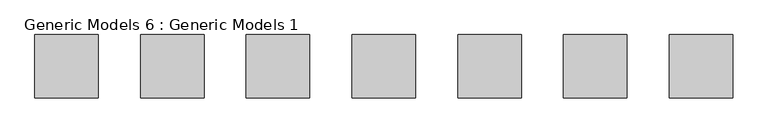
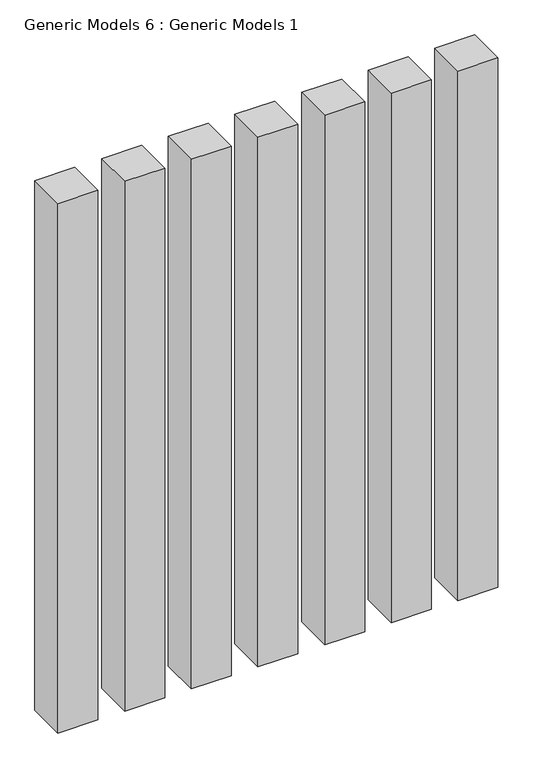
"""IFC4 building model written with IfcOpenShell, lengths in millimetres: proxy geometry, Generic Models 6 : Generic Models 1."""

from ifc_helpers import new_model, si_unit, origin, origin_with_axes, place, context, project, spatial, polyline, outline, extrude, source, transform, mapped, element, save


def generic_models_6_generic_models_1_46a45353(model_context):
    return source(origin(), model_context, "Body", "SweptSolid", [
        extrude(outline(polyline([(-9274.1453682, 14207.234892), (-9502.7453682, 14207.234892), (-9502.7453682, 14435.834892), (-9274.1453682, 14435.834892), (-9274.1453682, 14207.234892)])), origin_with_axes(), (0.0, 0.0, 1.0), 3200.4),
        extrude(outline(polyline([(-8893.1453682, 14207.234892), (-9121.7453682, 14207.234892), (-9121.7453682, 14435.834892), (-8893.1453682, 14435.834892), (-8893.1453682, 14207.234892)])), origin_with_axes(), (0.0, 0.0, 1.0), 3200.4),
        extrude(outline(polyline([(-8512.1453682, 14207.234892), (-8740.7453682, 14207.234892), (-8740.7453682, 14435.834892), (-8512.1453682, 14435.834892), (-8512.1453682, 14207.234892)])), origin_with_axes(), (0.0, 0.0, 1.0), 3200.4),
        extrude(outline(polyline([(-8131.1453682, 14207.234892), (-8359.7453682, 14207.234892), (-8359.7453682, 14435.834892), (-8131.1453682, 14435.834892), (-8131.1453682, 14207.234892)])), origin_with_axes(), (0.0, 0.0, 1.0), 3200.4),
        extrude(outline(polyline([(-7750.1453682, 14207.234892), (-7978.7453682, 14207.234892), (-7978.7453682, 14435.834892), (-7750.1453682, 14435.834892), (-7750.1453682, 14207.234892)])), origin_with_axes(), (0.0, 0.0, 1.0), 3200.4),
        extrude(outline(polyline([(-7369.1453682, 14207.234892), (-7597.7453682, 14207.234892), (-7597.7453682, 14435.834892), (-7369.1453682, 14435.834892), (-7369.1453682, 14207.234892)])), origin_with_axes(), (0.0, 0.0, 1.0), 3200.4),
        extrude(outline(polyline([(-6988.1453682, 14207.234892), (-7216.7453682, 14207.234892), (-7216.7453682, 14435.834892), (-6988.1453682, 14435.834892), (-6988.1453682, 14207.234892)])), origin_with_axes(), (0.0, 0.0, 1.0), 3200.4),
    ])


if __name__ == "__main__":
    model = new_model("IFC4")
    model_context = context("Model", 3, world=origin())
    ifc_project = project(units=[si_unit("LENGTHUNIT", "METRE", prefix="MILLI")], contexts=[model_context])
    site = spatial("IfcSite", under=ifc_project)
    building = spatial("IfcBuilding", under=site)
    placement = place(None, origin())
    generic_models_6_generic_models_1_shape = generic_models_6_generic_models_1_46a45353(model_context)
    element("IfcBuildingElementProxy", 1, Name="Generic Models 6 : Generic Models 1", ObjectType="Generic Models 6 : Generic Models 1", at=placement, inside=building, context=model_context, shape_type="MappedRepresentation", body=[
        mapped(generic_models_6_generic_models_1_shape, transform((0.0, 0.0, 0.0), x_axis=(1.0, 0.0, 0.0), y_axis=(0.0, 1.0, 0.0), z_axis=(0.0, 0.0, 1.0))),
    ])
    save(model, "model.ifc")

# Revit data of these elements
# Element 1 (IfcBuildingElementProxy, "Generic Models 6 : Generic Models 1")
#   Materials on its faces: "0 olive green"
# Materials
#   "0 olive green": class "Generic", colour RGB 120 120 120, transparency 0, Cost = 0
